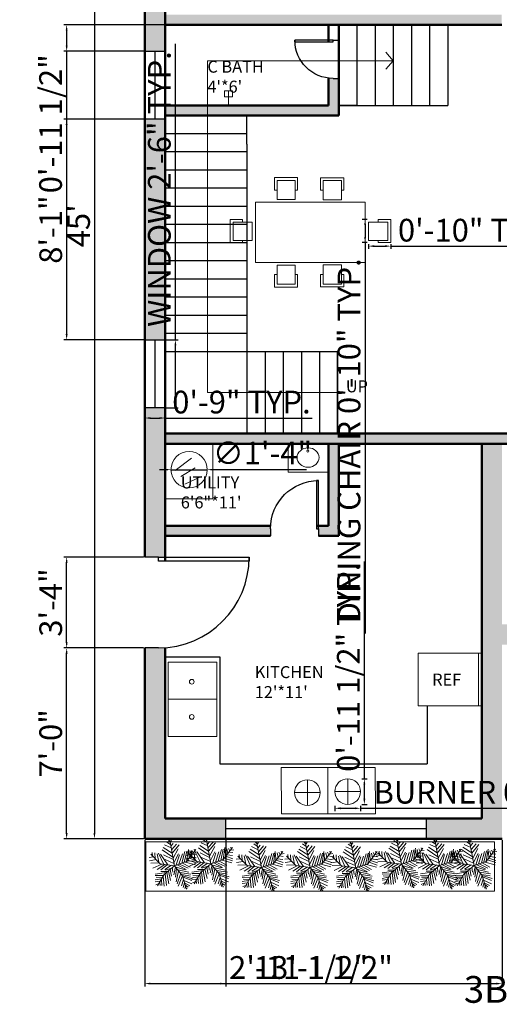
# Model space of a CAD drawing. Units: inches. Extents: x 772 to 1415, y 1573 to 2261.
# Tile 1 of 4: x 772 to 984, y 1573 to 2007. Entities that reach past the tile are written whole.
import ezdxf

# ---------------------------------------------------------------- set-up
doc = ezdxf.new("R2010")
doc.units = ezdxf.units.IN
for name, color, linetype, lineweight in [('A-ANNO-DIMS', 2, 'Continuous', 18), ('A-ANNO-SYMB', 7, 'Continuous', 18), ('A-ANNO-TEXT', 10, 'Continuous', 25), ('A-AREA-IDEN', 10, 'Continuous', 25), ('A-EQPM', 8, 'Continuous', 18), ('A-FLOR-FIXT', 9, 'Continuous', 18), ('A-FLOR-STRS', 7, 'Continuous', 25), ('A-FURN-FIXD', 210, 'Continuous', 25), ('A-WALL-PATT', 140, 'Continuous', 13), ('DOOR', 52, 'Continuous', 25), ('FUR', 210, 'Continuous', 18), ('L-PLNT-BEDS', 92, 'Continuous', 18), ('TREE', 92, 'Continuous', 13), ('WALL', 7, 'Continuous', 50), ('WINDOW', 80, 'Continuous', 25)]:
    doc.layers.add(name, color=color, linetype=linetype, lineweight=lineweight)
doc.styles.get("Standard").update_dxf_attribs({"font": 'arial.ttf'})
doc.dimstyles.new('ISO-25', dxfattribs={"dimtxt": 10, "dimasz": 2.5, "dimexe": 1.25, "dimexo": 0.625, "dimtad": 1, "dimdec": 0, "dimlunit": 4, "dimtxsty": 'Standard', "dimcen": 2.5, "dimadec": 0, "dimazin": 0, "dimtfac": 1, "dimtdec": 0, "dimtmove": 0, "dimatfit": 3, "dimfxl": 1, "dimarcsym": 0})

# ---------------------------------------------------------------- blocks, each defined once
blk = doc.blocks.new('*U2')
for p, q in [((0, 0), (0, -6)), ((40, 0), (40, -6))]:
    blk.add_line(p, q)
blk.add_lwpolyline([(0, 0), (0, 40), (1.75, 40), (1.75, 0)], close=True)
blk.add_arc((0, 0), 40, 0, 90)
blk = doc.blocks.new('*U6')
for p, q in [((-7.288, 39.707), (-21.778, 46.673)), ((-8.737, 47.138), (-17.069, 52.711)), ((-10.186, 53.64), (-13.084, 55.962)), ((0, 0), (-10.5, 57)), ((-9.099, 51.782), (-6.563, 55.962)), ((-7.65, 43.423), (-2.578, 49.46)), ((-5.839, 35.992), (4.667, 48.067)), ((-5.114, 27.632), (10.463, 46.673)), ((-31.5, 4.5), (-52.5, 25.5)), ((-48.585, 21.131), (-49.309, 29.026)), ((-43.513, 28.561), (-42.427, 15.558)), ((-38.442, 26.239), (-34.819, 7.663)), ((-35.544, 28.097), (-24.314, 3.947)), ((-14.533, 2.09), (-30.834, 25.31)), ((-3.665, 19.273), (-27.574, 35.527)), ((-5.114, 28.097), (-24.676, 40.636)), ((-24.314, 23.917), (-2.941, 13.7)), ((-2.941, 16.486), (8.652, 37.85)), ((-1.129, 6.734), (9.014, 26.704)), ((3.942, 1.625), (11.187, 24.381)), ((10.101, 3.483), (17.708, 26.239)), ((16.259, 5.805), (23.142, 31.348)), ((22.055, 7.198), (27.489, 32.277)), ((27, 9), (48, 36)), ((27.127, 9.056), (31.112, 35.992)), ((31.836, 30.883), (32.561, 16.486)), ((35.096, 32.741), (37.27, 22.524)), ((38.719, 34.134), (41.979, 28.561)), ((40.53, 25.775), (48.862, 24.846)), ((43.791, 29.954), (51.036, 30.883)), ((44.153, 36.456), (45.239, 32.741)), ((-47.498, 19.737), (-55.83, 18.344)), ((-40.615, 13.7), (-55.105, 10.913)), ((-33.37, 6.269), (-52.207, 5.34)), ((-28.299, 3.483), (-47.86, -5.805)), ((-21.416, 3.018), (-38.079, -8.128)), ((0, 0), (-31.5, 4.5)), ((-15.982, 2.09), (-30.11, -9.521)), ((0, 0), (-22.5, -19.5)), ((-6.563, 1.161), (-21.416, -8.128)), ((-20.691, 13.7), (-1.129, 4.876)), ((0, 0), (27, 9)), ((0, 0), (18, -22.5)), ((6.478, 1.625), (26.04, -8.592)), ((11.187, 3.483), (30.749, -5.805)), ((18.07, 5.805), (35.096, -3.483)), ((24.229, 7.663), (46.688, 1.625)), ((29.662, 12.307), (48.137, 6.269)), ((33.285, 16.486), (48.862, 10.913)), ((36.183, 19.737), (48.137, 17.88)), ((-17.431, -15.094), (-42.789, -18.809)), ((-24.314, -21.596), (-42.427, -22.06)), ((-22.5, -19.5), (-37.5, -45)), ((-15.257, -12.772), (-30.11, -12.772)), ((-20.691, -18.345), (-17.793, -44.352)), ((-6.563, -5.805), (-19.967, -9.985)), ((-17.069, -15.094), (-12.721, -40.172)), ((-13.446, -11.378), (-8.737, -32.741)), ((-9.461, -8.592), (-6.201, -23.453)), ((-4.752, -3.483), (-3.665, -14.629)), ((2.493, -3.019), (-1.491, -20.202)), ((1.769, -2.555), (24.229, -9.521)), ((5.029, -6.27), (2.131, -25.775)), ((9.014, -11.378), (3.58, -35.992)), ((14.085, -16.951), (6.478, -40.172)), ((7.565, -9.056), (32.198, -14.629)), ((12.274, -15.094), (36.907, -18.809)), ((16.259, -19.738), (36.183, -22.989)), ((-28.299, -29.026), (-42.789, -31.348)), ((-30.834, -34.135), (-42.427, -35.528)), ((-34.457, -39.708), (-40.978, -42.494)), ((-26.849, -26.24), (-40.253, -25.775)), ((-32.646, -36.921), (-31.921, -44.352)), ((-29.023, -30.884), (-27.936, -43.887)), ((-25.038, -23.918), (-22.865, -45.281)), ((18.07, -22.524), (8.289, -45.745)), ((20.244, -30.419), (15.897, -44.816)), ((18, -22.5), (27, -52.5)), ((18.433, -22.524), (40.53, -29.026)), ((19.157, -25.311), (38.719, -33.206)), ((22.78, -37.85), (19.519, -48.532)), ((21.331, -32.741), (39.081, -40.636)), ((22.78, -38.314), (34.372, -44.816)), ((24.591, -43.423), (30.749, -47.603)), ((24.591, -45.745), (23.142, -50.854)), ((26.764, -49.925), (28.213, -50.854))]:
    blk.add_line(p, q)
blk = doc.blocks.new('*D10')
at = {"layer": 'A-ANNO-DIMS', "color": 0, "lineweight": -2, "transparency": 16777216}
for p, q in [((827.03, 2185.98), (804.2, 2185.98)), ((805.45, 2183.48), (805.45, 1648.48)), ((827.03, 1645.98), (804.2, 1645.98))]:
    blk.add_line(p, q, dxfattribs=at)
at = {"layer": 'A-ANNO-DIMS', "color": 0, "transparency": 16777216}
for points in [[(805.04, 2183.48), (805.87, 2183.48), (805.45, 2185.98)], [(805.04, 1648.48), (805.87, 1648.48), (805.45, 1645.98)]]:
    blk.add_solid(points, dxfattribs=at)
at = {"layer": 'Defpoints', "color": 0, "transparency": 16777216}
for p in [(827.65, 2185.98), (805.45, 1645.98), (827.65, 1645.98)]:
    blk.add_point(p, dxfattribs=at)
at = {"layer": 'A-ANNO-DIMS', "color": 0, "transparency": 16777216, "insert": (799.74, 1915.98), "char_height": 10, "attachment_point": 5, "rotation": 90}
blk.add_mtext("45'", dxfattribs=at)
blk = doc.blocks.new('CHAIR-DINING')
for p, q in [((0, 4.23), (0, 9.75)), ((0, 9.75), (10.23, 9.75)), ((10.23, 9.75), (10.23, 4.23)), ((1.18, 4.23), (0, 4.23)), ((10.23, 4.23), (9.23, 4.23))]:
    blk.add_line(p, q)
blk.add_lwpolyline([(1.18, 0), (9.23, 0), (9.23, 8.46), (1.18, 8.46)], close=True)
blk = doc.blocks.new('WIN-88IN')
blk.add_line((0, 4.5), (88.26, 4.5))
blk.add_lwpolyline([(0, 9), (88.26, 9), (88.26, 0), (0, 0)], close=True)
blk = doc.blocks.new('WIN-30IN')
blk.add_line((4.5, 0), (4.5, 29.96))
blk.add_lwpolyline([(0, 29.96), (9, 29.96), (9, 0), (0, 0)], close=True)
blk = doc.blocks.new('COOKTOP-BURNER')
for p, q in [((5.65, 5.65), (5.65, 11.3)), ((5.65, 11.3), (5.65, 0)), ((11.3, 5.65), (0, 5.65)), ((5.65, 0), (5.65, 5.65)), ((5.65, 5.65), (11.3, 5.65))]:
    blk.add_line(p, q)
blk.add_circle((5.65, 5.65), 5.65)
blk = doc.blocks.new('*D25')
at = {"layer": 'A-ANNO-DIMS', "color": 0, "lineweight": -2, "transparency": 16777216}
for p, q in [((925.67, 1918.77), (923.51, 1918.77)), ((924.76, 1916.27), (924.76, 1911.03)), ((925.67, 1908.53), (923.51, 1908.53)), ((924.76, 1908.53), (924.76, 1736.44))]:
    blk.add_line(p, q, dxfattribs=at)
at = {"layer": 'A-ANNO-DIMS', "color": 0, "transparency": 16777216}
for points in [[(924.34, 1916.27), (925.17, 1916.27), (924.76, 1918.77)], [(924.34, 1911.03), (925.17, 1911.03), (924.76, 1908.53)]]:
    blk.add_solid(points, dxfattribs=at)
at = {"layer": 'Defpoints', "color": 0, "transparency": 16777216}
for p in [(926.29, 1918.77), (924.76, 1908.53), (926.29, 1908.53)]:
    blk.add_point(p, dxfattribs=at)
at = {"layer": 'A-ANNO-DIMS', "color": 0, "transparency": 16777216, "insert": (918.96, 1821.24), "char_height": 10, "attachment_point": 5, "rotation": 90}
blk.add_mtext('DINING CHAIR 0\'-10" TYP.', dxfattribs=at)
blk = doc.blocks.new('*D26')
at = {"layer": 'A-ANNO-DIMS', "color": 0, "lineweight": -2, "transparency": 16777216}
for p, q in [((926.29, 1907.91), (926.29, 1905.75)), ((928.79, 1907), (933.54, 1907)), ((936.04, 1907.91), (936.04, 1905.75)), ((936.04, 1907), (1008.52, 1907))]:
    blk.add_line(p, q, dxfattribs=at)
at = {"layer": 'A-ANNO-DIMS', "color": 0, "transparency": 16777216}
for points in [[(928.79, 1907.42), (928.79, 1906.58), (926.29, 1907)], [(933.54, 1907.42), (933.54, 1906.58), (936.04, 1907)]]:
    blk.add_solid(points, dxfattribs=at)
at = {"layer": 'Defpoints', "color": 0, "transparency": 16777216}
for p in [(926.29, 1908.53), (936.04, 1908.53), (936.04, 1907)]:
    blk.add_point(p, dxfattribs=at)
at = {"layer": 'A-ANNO-DIMS', "color": 0, "transparency": 16777216, "insert": (973.53, 1912.73), "char_height": 10, "attachment_point": 5}
blk.add_mtext('0\'-10" TYP.', dxfattribs=at)
blk = doc.blocks.new('*D35')
at = {"layer": 'A-ANNO-DIMS', "color": 0, "lineweight": -2, "transparency": 16777216}
for p, q in [((841.15, 1865.74), (841.15, 1996.03)), ((837.28, 1865.74), (842.4, 1865.74)), ((841.15, 1838.28), (841.15, 1863.24)), ((837.28, 1835.78), (842.4, 1835.78))]:
    blk.add_line(p, q, dxfattribs=at)
at = {"layer": 'A-ANNO-DIMS', "color": 0, "transparency": 16777216}
for points in [[(840.73, 1863.24), (841.56, 1863.24), (841.15, 1865.74)], [(840.73, 1838.28), (841.56, 1838.28), (841.15, 1835.78)]]:
    blk.add_solid(points, dxfattribs=at)
at = {"layer": 'Defpoints', "color": 0, "transparency": 16777216}
for p in [(836.65, 1865.74), (841.15, 1865.74), (836.65, 1835.78)]:
    blk.add_point(p, dxfattribs=at)
at = {"layer": 'A-ANNO-DIMS', "color": 0, "transparency": 16777216, "insert": (835.35, 1932.14), "char_height": 10, "attachment_point": 5, "rotation": 90}
blk.add_mtext('WINDOW 2\'-6" TYP.', dxfattribs=at)
blk = doc.blocks.new('*D36')
at = {"layer": 'A-ANNO-DIMS', "color": 0, "lineweight": -2, "transparency": 16777216}
for p, q in [((827.65, 1835.15), (827.65, 1830.04)), ((836.65, 1835.15), (836.65, 1830.04)), ((830.15, 1831.29), (834.15, 1831.29)), ((836.65, 1831.29), (901.36, 1831.29))]:
    blk.add_line(p, q, dxfattribs=at)
at = {"layer": 'A-ANNO-DIMS', "color": 0, "transparency": 16777216}
for points in [[(830.15, 1831.7), (830.15, 1830.87), (827.65, 1831.29)], [(834.15, 1831.7), (834.15, 1830.87), (836.65, 1831.29)]]:
    blk.add_solid(points, dxfattribs=at)
at = {"layer": 'Defpoints', "color": 0, "transparency": 16777216}
for p in [(827.65, 1835.78), (836.65, 1835.78), (836.65, 1831.29)]:
    blk.add_point(p, dxfattribs=at)
at = {"layer": 'A-ANNO-DIMS', "color": 0, "transparency": 16777216, "insert": (870.25, 1837.02), "char_height": 10, "attachment_point": 5}
blk.add_mtext('0\'-9" TYP.', dxfattribs=at)
blk = doc.blocks.new('*D39')
at = {"layer": 'A-ANNO-DIMS', "color": 0, "lineweight": -2, "transparency": 16777216}
for p, q in [((911.44, 1660.47), (911.44, 1658.15)), ((913.94, 1659.4), (920.23, 1659.4)), ((922.73, 1660.47), (922.73, 1658.15)), ((922.73, 1659.4), (1080.94, 1659.4))]:
    blk.add_line(p, q, dxfattribs=at)
at = {"layer": 'A-ANNO-DIMS', "color": 0, "transparency": 16777216}
for points in [[(913.94, 1659.82), (913.94, 1658.99), (911.44, 1659.4)], [(920.23, 1659.82), (920.23, 1658.99), (922.73, 1659.4)]]:
    blk.add_solid(points, dxfattribs=at)
at = {"layer": 'Defpoints', "color": 0, "transparency": 16777216}
for p in [(911.44, 1661.1), (922.73, 1661.1), (922.73, 1659.4)]:
    blk.add_point(p, dxfattribs=at)
at = {"layer": 'A-ANNO-DIMS', "color": 0, "transparency": 16777216, "insert": (1003.09, 1665.2), "char_height": 10, "attachment_point": 5}
blk.add_mtext('BURNER 0\'-11 1/2" TYP.', dxfattribs=at)
blk = doc.blocks.new('*D40')
at = {"layer": 'A-ANNO-DIMS', "color": 0, "lineweight": -2, "transparency": 16777216}
for p, q in [((924.43, 1672.4), (924.43, 1768.17)), ((923.36, 1672.4), (925.68, 1672.4)), ((924.43, 1663.6), (924.43, 1669.9)), ((923.36, 1661.1), (925.68, 1661.1))]:
    blk.add_line(p, q, dxfattribs=at)
at = {"layer": 'A-ANNO-DIMS', "color": 0, "transparency": 16777216}
for points in [[(924.01, 1669.9), (924.85, 1669.9), (924.43, 1672.4)], [(924.01, 1663.6), (924.85, 1663.6), (924.43, 1661.1)]]:
    blk.add_solid(points, dxfattribs=at)
at = {"layer": 'Defpoints', "color": 0, "transparency": 16777216}
for p in [(922.73, 1672.4), (924.43, 1672.4), (922.73, 1661.1)]:
    blk.add_point(p, dxfattribs=at)
at = {"layer": 'A-ANNO-DIMS', "color": 0, "transparency": 16777216, "insert": (918.63, 1721.54), "char_height": 10, "attachment_point": 5, "rotation": 90}
blk.add_mtext('0\'-11 1/2" TYP.', dxfattribs=at)
blk = doc.blocks.new('*D41')
at = {"layer": 'A-ANNO-DIMS', "color": 0, "lineweight": -2, "transparency": 16777216}
for p, q in [((827.65, 1645.36), (827.65, 1580.94)), ((985.15, 1645.36), (985.15, 1580.94)), ((830.15, 1582.19), (982.65, 1582.19))]:
    blk.add_line(p, q, dxfattribs=at)
at = {"layer": 'A-ANNO-DIMS', "color": 0, "transparency": 16777216}
for points in [[(830.15, 1582.61), (830.15, 1581.78), (827.65, 1582.19)], [(982.65, 1582.61), (982.65, 1581.78), (985.15, 1582.19)]]:
    blk.add_solid(points, dxfattribs=at)
at = {"layer": 'Defpoints', "color": 0, "transparency": 16777216}
for p in [(827.65, 1645.98), (985.15, 1645.98), (985.15, 1582.19)]:
    blk.add_point(p, dxfattribs=at)
at = {"layer": 'A-ANNO-DIMS', "color": 0, "transparency": 16777216, "insert": (906.4, 1587.99), "char_height": 10, "attachment_point": 5}
blk.add_mtext('13\'-1 1/2"', dxfattribs=at)
blk = doc.blocks.new('*D52')
at = {"layer": 'A-ANNO-DIMS', "color": 0, "lineweight": -2, "transparency": 16777216}
for p, q in [((836.03, 2004.48), (791.95, 2004.48)), ((793.2, 2001.98), (793.2, 1995.35)), ((827.03, 1992.85), (791.95, 1992.85)), ((793.2, 1992.85), (793.2, 1931.44))]:
    blk.add_line(p, q, dxfattribs=at)
at = {"layer": 'A-ANNO-DIMS', "color": 0, "transparency": 16777216}
for points in [[(792.78, 2001.98), (793.62, 2001.98), (793.2, 2004.48)], [(792.78, 1995.35), (793.62, 1995.35), (793.2, 1992.85)]]:
    blk.add_solid(points, dxfattribs=at)
at = {"layer": 'Defpoints', "color": 0, "transparency": 16777216}
for p in [(836.65, 2004.48), (793.2, 1992.85), (827.65, 1992.85)]:
    blk.add_point(p, dxfattribs=at)
at = {"layer": 'A-ANNO-DIMS', "color": 0, "transparency": 16777216, "insert": (787.4, 1960.9), "char_height": 10, "attachment_point": 5, "rotation": 90}
blk.add_mtext('0\'-11 1/2"', dxfattribs=at)
blk = doc.blocks.new('*D53')
at = {"layer": 'A-ANNO-DIMS', "color": 0, "lineweight": -2, "transparency": 16777216}
for p, q in [((827.03, 1962.89), (791.95, 1962.89)), ((793.2, 1960.39), (793.2, 1868.24)), ((827.03, 1865.74), (791.95, 1865.74))]:
    blk.add_line(p, q, dxfattribs=at)
at = {"layer": 'A-ANNO-DIMS', "color": 0, "transparency": 16777216}
for points in [[(792.78, 1960.39), (793.62, 1960.39), (793.2, 1962.89)], [(792.78, 1868.24), (793.62, 1868.24), (793.2, 1865.74)]]:
    blk.add_solid(points, dxfattribs=at)
at = {"layer": 'Defpoints', "color": 0, "transparency": 16777216}
for p in [(827.65, 1962.89), (793.2, 1865.74), (827.65, 1865.74)]:
    blk.add_point(p, dxfattribs=at)
at = {"layer": 'A-ANNO-DIMS', "color": 0, "transparency": 16777216, "insert": (787.47, 1914.31), "char_height": 10, "attachment_point": 5, "rotation": 90}
blk.add_mtext('8\'-1"', dxfattribs=at)
blk = doc.blocks.new('*D54')
at = {"layer": 'A-ANNO-DIMS', "color": 0, "lineweight": -2, "transparency": 16777216}
for p, q in [((827.65, 1645.36), (827.65, 1580.94)), ((863.4, 1645.36), (863.4, 1580.94)), ((830.15, 1582.19), (860.9, 1582.19)), ((863.4, 1582.19), (924.97, 1582.19))]:
    blk.add_line(p, q, dxfattribs=at)
at = {"layer": 'A-ANNO-DIMS', "color": 0, "transparency": 16777216}
for points in [[(830.15, 1582.61), (830.15, 1581.78), (827.65, 1582.19)], [(860.9, 1582.61), (860.9, 1581.78), (863.4, 1582.19)]]:
    blk.add_solid(points, dxfattribs=at)
at = {"layer": 'Defpoints', "color": 0, "transparency": 16777216}
for p in [(827.65, 1645.98), (863.4, 1645.98), (863.4, 1582.19)]:
    blk.add_point(p, dxfattribs=at)
at = {"layer": 'A-ANNO-DIMS', "color": 0, "transparency": 16777216, "insert": (895.44, 1587.99), "char_height": 10, "attachment_point": 5}
blk.add_mtext('2\'-11 1/2"', dxfattribs=at)
blk = doc.blocks.new('*D57')
at = {"layer": 'A-ANNO-DIMS', "color": 0, "lineweight": -2, "transparency": 16777216}
for p, q in [((827.03, 1730.04), (791.95, 1730.04)), ((793.2, 1648.48), (793.2, 1727.54)), ((827.03, 1645.98), (791.95, 1645.98))]:
    blk.add_line(p, q, dxfattribs=at)
at = {"layer": 'A-ANNO-DIMS', "color": 0, "transparency": 16777216}
for points in [[(792.78, 1727.54), (793.62, 1727.54), (793.2, 1730.04)], [(792.78, 1648.48), (793.62, 1648.48), (793.2, 1645.98)]]:
    blk.add_solid(points, dxfattribs=at)
at = {"layer": 'Defpoints', "color": 0, "transparency": 16777216}
for p in [(793.2, 1730.04), (827.65, 1730.04), (827.65, 1645.98)]:
    blk.add_point(p, dxfattribs=at)
at = {"layer": 'A-ANNO-DIMS', "color": 0, "transparency": 16777216, "insert": (787.47, 1688.01), "char_height": 10, "attachment_point": 5, "rotation": 90}
blk.add_mtext('7\'-0"', dxfattribs=at)
blk = doc.blocks.new('*D58')
at = {"layer": 'A-ANNO-DIMS', "color": 0, "lineweight": -2, "transparency": 16777216}
for p, q in [((827.03, 1770.04), (791.95, 1770.04)), ((793.2, 1732.54), (793.2, 1767.54)), ((827.03, 1730.04), (791.95, 1730.04))]:
    blk.add_line(p, q, dxfattribs=at)
at = {"layer": 'A-ANNO-DIMS', "color": 0, "transparency": 16777216}
for points in [[(792.78, 1767.54), (793.62, 1767.54), (793.2, 1770.04)], [(792.78, 1732.54), (793.62, 1732.54), (793.2, 1730.04)]]:
    blk.add_solid(points, dxfattribs=at)
at = {"layer": 'Defpoints', "color": 0, "transparency": 16777216}
for p in [(793.2, 1770.04), (827.65, 1770.04), (827.65, 1730.04)]:
    blk.add_point(p, dxfattribs=at)
at = {"layer": 'A-ANNO-DIMS', "color": 0, "transparency": 16777216, "insert": (787.47, 1750.04), "char_height": 10, "attachment_point": 5, "rotation": 90}
blk.add_mtext('3\'-4"', dxfattribs=at)
blk = doc.blocks.new('*D67')
at = {"layer": 'A-ANNO-DIMS', "color": 0, "lineweight": -2, "transparency": 16777216}
for p, q in [((836.67, 1808.54), (834.17, 1808.54)), ((839.17, 1808.54), (855.18, 1808.54)), ((898.89, 1808.54), (857.68, 1808.54))]:
    blk.add_line(p, q, dxfattribs=at)
at = {"layer": 'A-ANNO-DIMS', "color": 0, "transparency": 16777216}
for points in [[(836.67, 1808.96), (836.67, 1808.13), (839.17, 1808.54)], [(857.68, 1808.96), (857.68, 1808.13), (855.18, 1808.54)]]:
    blk.add_solid(points, dxfattribs=at)
at = {"layer": 'Defpoints', "color": 0, "transparency": 16777216}
for p in [(839.17, 1808.54), (855.18, 1808.54)]:
    blk.add_point(p, dxfattribs=at)
at = {"layer": 'A-ANNO-DIMS', "color": 0, "transparency": 16777216, "insert": (879.53, 1814.55), "char_height": 10, "attachment_point": 5, "rotation": 359.9994}
blk.add_mtext('∅1\'-4"', dxfattribs=at)

msp = doc.modelspace()

# ---------------------------------------------------------------- hatches: boundary and pattern name
at = {"layer": 'A-WALL-PATT'}
h = msp.add_hatch(color=256, dxfattribs=at)
h.dxf.hatch_style = 1
h.paths.add_polyline_path([(885.72, 2185.98), (827.65, 2185.98), (827.65, 1992.85), (836.65, 1992.85), (836.65, 2176.98), (885.72, 2176.98)])
h.paths.add_polyline_path([(1050.98, 2185.98), (977.81, 2185.98), (977.81, 2176.98), (1028.65, 2176.98), (1050.98, 2176.98)])
h.paths.add_polyline_path([(1112.88, 2185.98), (1085.61, 2185.98), (1085.61, 2176.98), (1105.15, 2176.98), (1112.88, 2176.98)])
h.paths.add_polyline_path([(1192.68, 2185.98), (1147.51, 2185.98), (1147.51, 2176.98), (1181.65, 2176.98), (1192.68, 2176.98)])
h.paths.add_polyline_path([(1307.65, 2185.98), (1284.78, 2185.98), (1284.78, 2176.98), (1298.65, 2176.98), (1298.65, 1819.98), (1307.65, 1819.98)])
h.paths.add_polyline_path([(1033.15, 2176.98), (1028.65, 2176.98), (1028.65, 2036.41), (1032.25, 2036.41, -0.009373), (1033.15, 2036.4)])
h.paths.add_polyline_path([(1036.22, 2092.98), (1033.15, 2092.98), (1033.15, 2088.48), (1036.22, 2088.48)])
h.paths.add_polyline_path([(1154.65, 2104.98), (1135.16, 2104.98, -0.008763), (1135.17, 2104.13), (1135.17, 2100.48), (1154.65, 2100.48)])
h.paths.add_polyline_path([(1159.15, 2176.98), (1154.65, 2176.98), (1154.65, 2051.78), (1159.15, 2051.78)])
h.paths.add_polyline_path([(914.37, 1839.72), (927.25, 1839.72), (927.25, 1850.6), (914.37, 1850.6)], flags=9)
h.paths.add_polyline_path([(1081.37, 1890.08), (1108.45, 1890.08), (1108.45, 1909.77), (1081.37, 1909.77)], flags=9)
h.paths.add_polyline_path([(1220.18, 1938.14), (1269.92, 1938.14), (1269.92, 1957.83), (1220.18, 1957.83)], flags=9)
h.paths.add_polyline_path([(1219.66, 2046.23), (1263.24, 2046.23), (1263.24, 2065.92), (1219.66, 2065.92)], flags=9)
h.paths.add_polyline_path([(1107.96, 2127.66), (1143.78, 2127.66), (1143.78, 2147.35), (1107.96, 2147.35)], flags=9)
h.paths.add_polyline_path([(1040.84, 2046.02), (1081.99, 2046.02), (1081.99, 2065.72), (1040.84, 2065.72)], flags=9)
h.paths.add_polyline_path([(1051.44, 2131.75), (1073.61, 2131.75), (1073.61, 2151.44), (1051.44, 2151.44)], flags=9)
h.paths.add_polyline_path([(953.87, 2096.26), (1003.05, 2096.26), (1003.05, 2115.95), (953.87, 2115.95)], flags=9)
h = msp.add_hatch(color=256, dxfattribs=at)
h.dxf.hatch_style = 1
h.paths.add_polyline_path([(836.65, 1835.78), (827.65, 1835.78), (827.65, 1770.04), (833.65, 1770.04), (836.65, 1770.04)])
h.paths.add_polyline_path([(1154.65, 1824.48), (938.65, 1824.48), (836.65, 1824.48), (836.65, 1819.98), (980.65, 1819.98), (1154.65, 1819.98)])
h.paths.add_polyline_path([(836.65, 1962.89), (827.65, 1962.89), (827.65, 1865.74), (836.65, 1865.74)])
h.paths.add_polyline_path([(913.15, 1980.86), (910.62, 1980.86, -0.029352), (908.65, 1980.98), (908.65, 1968.98), (900.27, 1968.98), (855.22, 1968.98), (855.22, 1964.48), (913.15, 1964.48)])
h.paths.add_polyline_path([(855.22, 1968.98), (836.65, 1968.98), (836.65, 1964.48), (855.22, 1964.48)])
h.paths.add_polyline_path([(984.95, 2008.98), (836.65, 2008.98), (836.65, 2004.48), (908.65, 2004.48), (984.95, 2004.48)])
h.paths.add_polyline_path([(1298.65, 2008.98), (1171.7, 2008.98), (1154.65, 2008.98), (1154.65, 2004.48), (1298.65, 2004.48)])
h.paths.add_polyline_path([(1159.15, 2011.78), (1154.65, 2011.78), (1154.65, 2008.98), (1159.15, 2008.98)])
h.paths.add_polyline_path([(1159.15, 2004.48), (1154.65, 2004.48), (1154.65, 1998.53), (1159.15, 1998.53)])
h = msp.add_hatch(color=256, dxfattribs=at)
h.dxf.hatch_style = 1
h.paths.add_polyline_path([(863.4, 1654.98), (836.65, 1654.98), (836.65, 1678.98), (836.65, 1730.15, -0.01877), (833.65, 1730.04), (827.65, 1730.04), (827.65, 1645.98), (863.4, 1645.98)])
h.paths.add_polyline_path([(985.15, 1654.98), (985.15, 1819.98), (976.15, 1819.98), (976.15, 1654.98), (951.66, 1654.98), (951.66, 1645.98), (985.15, 1645.98)])
h.paths.add_polyline_path([(989, 1737.48), (989, 1740.48), (985.15, 1740.48), (985.15, 1731.48), (989, 1731.48)])
h.paths.add_polyline_path([(1045.2, 1740.48), (1028.89, 1740.48, -0.01877), (1029, 1737.48), (1029, 1731.48), (1045.2, 1731.48)])
h.paths.add_polyline_path([(1145.65, 1819.98), (1136.65, 1819.98), (1136.65, 1740.48), (1133.46, 1740.48), (1133.46, 1731.48), (1145.65, 1731.48)])
h = msp.add_hatch(color=256, dxfattribs=at)
h.dxf.hatch_style = 1
h.paths.add_polyline_path([(883.08, 1783.87), (836.65, 1783.87), (836.65, 1779.37), (883.04, 1779.37), (883.04, 1782.55, -0.015579)])
h.paths.add_polyline_path([(913.15, 1819.98), (908.65, 1819.98), (908.65, 1807.38), (908.65, 1783.87), (904.24, 1783.87), (904.24, 1782.55), (904.24, 1779.37), (913.15, 1779.37)])

# ---------------------------------------------------------------- linework, layer by layer
at = {"layer": 'A-ANNO-SYMB'}
for p, q in [((937.15, 1988.68), (933.87, 1992.46)), ((855.22, 1842.48), (855.22, 1988.68)), ((855.22, 1988.68), (937.15, 1988.68)), ((937.15, 1988.68), (933.87, 1984.9)), ((912.63, 1842.48), (855.22, 1842.48))]:
    msp.add_line(p, q, dxfattribs=at)
at = {"layer": 'A-EQPM'}
for p, q in [((841.01, 1808.21), (848.29, 1813.6)), ((843.51, 1805.55), (849.84, 1809.43)), ((845.29, 1802.11), (852.51, 1805.6)), ((974.79, 1727.66), (974.79, 1704.52)), ((908.3, 1677.32), (908.3, 1656.94))]:
    msp.add_line(p, q, dxfattribs=at)
for points in [[(836.65, 1819.98), (857.6, 1819.98), (857.6, 1795.77), (836.65, 1795.77)], [(976.15, 1727.66), (948.12, 1727.66), (948.12, 1704.52), (976.15, 1704.52)], [(887.81, 1677.32), (929.23, 1677.32), (929.28, 1656.94), (887.86, 1656.94)]]:
    msp.add_lwpolyline(points, close=True, dxfattribs=at)
msp.add_circle((847.18, 1808.54), 8, dxfattribs=at)
at = {"layer": 'A-FLOR-FIXT'}
for p, q in [((864.52, 1975.46), (864.52, 1968.98)), ((837.9, 1707.4), (859.33, 1707.4))]:
    msp.add_line(p, q, dxfattribs=at)
for points in [[(862.75, 1972.76), (866.28, 1972.76), (866.28, 1975.46), (862.75, 1975.46)], [(908.65, 1819.98), (890.87, 1819.98), (890.87, 1807.38), (908.65, 1807.38)], [(837.9, 1723.81), (859.33, 1723.81), (859.33, 1691), (837.9, 1691)]]:
    msp.add_lwpolyline(points, close=True, dxfattribs=at)
for centre, radius in [((899.53, 1816.76), 0.441), ((848.37, 1715.15), 1.03), ((848.37, 1699.63), 1.03)]:
    msp.add_circle(centre, radius, dxfattribs=at)
msp.add_ellipse((899.64, 1813.89), major_axis=(4.86, 0), ratio=0.875, dxfattribs=at)
at = {"layer": 'A-FLOR-STRS'}
for p, q in [((921.15, 2004.48), (921.15, 1968.98)), ((929.15, 2004.48), (929.15, 1968.98)), ((937.15, 2004.48), (937.15, 1968.98)), ((945.15, 2004.48), (945.15, 1968.98)), ((953.15, 2004.48), (953.15, 1968.98)), ((961.15, 2004.48), (961.15, 1968.98)), ((921.15, 1968.98), (913.15, 1968.98)), ((913.15, 1968.98), (961.15, 1968.98)), ((872.65, 1964.48), (836.65, 1964.48)), ((872.65, 1951.98), (872.65, 1964.48)), ((872.65, 1956.48), (836.65, 1956.48)), ((872.65, 1951.98), (872.65, 1860.48)), ((872.65, 1948.48), (836.65, 1948.48)), ((872.65, 1940.48), (836.65, 1940.48)), ((872.65, 1932.48), (836.65, 1932.48)), ((872.65, 1924.48), (836.65, 1924.48)), ((872.65, 1916.48), (836.65, 1916.48)), ((872.65, 1908.48), (836.65, 1908.48)), ((872.65, 1900.48), (836.65, 1900.48)), ((872.65, 1892.48), (836.65, 1892.48)), ((872.65, 1884.48), (836.65, 1884.48)), ((872.65, 1876.48), (836.65, 1876.48)), ((872.65, 1868.48), (836.65, 1868.48)), ((872.65, 1860.48), (836.65, 1860.48)), ((912.63, 1860.48), (872.65, 1860.48)), ((872.65, 1860.48), (872.65, 1824.48)), ((880.65, 1860.48), (880.65, 1824.48)), ((888.65, 1860.48), (888.65, 1824.48)), ((896.65, 1860.48), (896.65, 1824.48)), ((904.65, 1860.48), (904.65, 1824.48)), ((912.63, 1824.48), (912.63, 1860.48)), ((912.65, 1860.48), (912.65, 1824.48))]:
    msp.add_line(p, q, dxfattribs=at)
at = {"layer": 'A-FURN-FIXD'}
for p, q in [((836.65, 1726.06), (836.65, 1726.06)), ((836.65, 1726.06), (860.65, 1726.06)), ((860.65, 1726.06), (860.65, 1678.98)), ((952.15, 1704.52), (952.15, 1678.98)), ((836.65, 1654.98), (836.65, 1678.98)), ((860.65, 1678.98), (952.15, 1678.98))]:
    msp.add_line(p, q, dxfattribs=at)
at = {"layer": 'FUR'}
msp.add_lwpolyline([(876.47, 1926.34), (924.81, 1926.34), (924.81, 1899.83), (876.47, 1899.83)], close=True, dxfattribs=at)
at = {"layer": 'L-PLNT-BEDS'}
msp.add_lwpolyline([(828.15, 1644.58), (981.82, 1644.58), (981.82, 1622.85), (828.15, 1622.85)], close=True, dxfattribs=at)
at = {"layer": 'WALL'}
for p, q in [((827.65, 1770.04), (827.65, 2185.98)), ((836.65, 1768.29), (836.65, 2176.98)), ((836.65, 2004.48), (908.65, 2004.48)), ((984.95, 2004.48), (836.65, 2004.48)), ((908.65, 1999.98), (908.65, 2004.48)), ((913.15, 1999.98), (913.15, 2004.48)), ((908.65, 1999.98), (908.65, 1996.97)), ((913.15, 1999.98), (913.15, 1997.71)), ((913.15, 1999.98), (913.15, 1964.48)), ((908.65, 1968.98), (908.65, 1980.98)), ((913.15, 1968.98), (913.15, 1980.86)), ((900.27, 1968.98), (836.65, 1968.98)), ((908.65, 1968.98), (900.27, 1968.98)), ((913.15, 1969.61), (913.15, 1966.48)), ((913.15, 1964.48), (913.15, 1968.98)), ((913.15, 1964.48), (836.65, 1964.48)), ((938.65, 1824.48), (836.65, 1824.48)), ((1154.65, 1824.48), (938.65, 1824.48)), ((1154.65, 1819.98), (836.65, 1819.98)), ((836.65, 1819.98), (980.65, 1819.98)), ((836.65, 1819.98), (836.65, 1783.98)), ((908.65, 1783.87), (908.65, 1819.98)), ((913.15, 1779.37), (913.15, 1819.98)), ((976.15, 1819.98), (976.15, 1654.98)), ((836.65, 1783.87), (883.08, 1783.87)), ((903.31, 1783.87), (908.65, 1783.87)), ((836.65, 1779.37), (883.04, 1779.37)), ((904.24, 1779.37), (913.15, 1779.37)), ((827.65, 1645.98), (827.65, 1730.04)), ((836.65, 1654.98), (836.65, 1730.15)), ((976.15, 1654.98), (836.65, 1654.98)), ((985.15, 1645.98), (827.65, 1645.98))]:
    msp.add_line(p, q, dxfattribs=at)

# ---------------------------------------------------------------- block references
at = {"layer": 'A-EQPM'}
for p in [(893.66, 1660.67), (911.44, 1661.1)]:
    msp.add_blockref('COOKTOP-BURNER', p, dxfattribs=at)
at = {"layer": 'DOOR', "xscale": -0.42118038010609, "yscale": 0.42118038010609, "zscale": 0.42118038010609, "rotation": 90}
msp.add_blockref('*U2', (910.62, 1997.71), dxfattribs=at)
at = {"layer": 'DOOR', "xscale": -0.5299835864931757, "yscale": 0.5299835864931757, "zscale": 0.5299835864931757}
msp.add_blockref('*U2', (904.24, 1782.55), dxfattribs=at)
at = {"layer": 'DOOR', "rotation": 270}
msp.add_blockref('*U2', (833.65, 1770.04), dxfattribs=at)
at = {"layer": 'FUR'}
for p in [(884.75, 1927.48), (905.12, 1927.39)]:
    msp.add_blockref('CHAIR-DINING', p, dxfattribs=at)
at = {"layer": 'FUR', "extrusion": (0, 0, -1), "zscale": -1}
for p, rotation in [((-874.99, 1918.77), 270.0000000000017), ((-884.75, 1898.69), 180), ((-905.12, 1898.77), 180)]:
    msp.add_blockref('CHAIR-DINING', p, dxfattribs=dict(at, rotation=rotation))
at = {"layer": 'FUR', "rotation": 270.000000000001}
msp.add_blockref('CHAIR-DINING', (926.29, 1918.77), dxfattribs=at)
at = {"layer": 'TREE', "xscale": 0.198069497027702, "yscale": 0.198069497027702, "zscale": 0.198069497027702}
for p in [(840.69, 1634.12), (856.8, 1635.01), (879.02, 1633.31), (900.47, 1633.31), (920.6, 1633.18), (940.74, 1634.75), (957.6, 1634.23), (972.77, 1634.23)]:
    msp.add_blockref('*U6', p, dxfattribs=at)
at = {"layer": 'WINDOW'}
for name, p in [('WIN-30IN', (827.65, 1962.89)), ('WIN-30IN', (827.65, 1835.78)), ('WIN-88IN', (863.4, 1645.98))]:
    msp.add_blockref(name, p, dxfattribs=at)

# ---------------------------------------------------------------- texts
at = {"layer": 'A-ANNO-TEXT', "attachment_point": 1}
for s, width, gutter_width, insert, char_height in [('UP', 83.1931, 26.39, (916.27, 1847.88), 5.277), ('REF', 83.1931, 26.39, (954.31, 1718.74), 5.277), ('3BHK HOUSE PLAN', 1239.311, 58.94, (968.3, 1585.54), 11.7878)]:
    msp.add_mtext_dynamic_manual_height_columns(s, width=width, gutter_width=gutter_width, heights=[0], dxfattribs=dict(at, insert=insert, char_height=char_height))
at = {"layer": 'A-AREA-IDEN', "char_height": 5.277, "attachment_point": 1}
for s, insert in [("C BATH\\P4'*6'", (855.22, 1988.68)), ('UTILITY\\P6\'6"*11\'', (843.51, 1805.55)), ("KITCHEN\\P12'*11'", (876.11, 1722.02))]:
    msp.add_mtext_dynamic_manual_height_columns(s, width=83.1931, gutter_width=26.39, heights=[0], dxfattribs=dict(at, insert=insert))

# ---------------------------------------------------------------- dimensions: what is measured, and where the dimension line sits
at = {"layer": 'A-ANNO-DIMS'}
for base, p1, p2, override, picture, middle in [((805.45, 1645.98), (827.65, 2185.98), (827.65, 1645.98), {"dimclrd": 0, "dimclre": 0, "dimclrt": 0}, '*D10', (799.74, 1915.98)), ((793.2, 1992.85), (836.65, 2004.48), (827.65, 1992.85), {"dimdec": 1, "dimlfac": 1, "dimrnd": 0, "dimzin": 1, "dimdsep": 46, "dimlunit": 4, "dimfrac": 2}, '*D52', (787.4, 1960.9)), ((793.1995, 1865.7405), (827.6509, 1962.8864), (827.6509, 1865.7405), {"dimdec": 1, "dimlfac": 1, "dimrnd": 0, "dimzin": 1, "dimdsep": 46, "dimlunit": 4, "dimfrac": 2}, '*D53', (787.4687, 1914.3134)), ((793.2, 1770.04), (827.65, 1730.04), (827.65, 1770.04), {"dimdec": 1, "dimlfac": 1, "dimrnd": 0, "dimzin": 1, "dimdsep": 46, "dimlunit": 4, "dimfrac": 2}, '*D58', (787.47, 1750.04)), ((793.2, 1730.04), (827.65, 1645.98), (827.65, 1730.04), {"dimdec": 1, "dimlfac": 1, "dimrnd": 0, "dimzin": 1, "dimdsep": 46, "dimlunit": 4, "dimfrac": 2}, '*D57', (787.47, 1688.01))]:
    dim = msp.add_linear_dim(base=base, p1=p1, p2=p2, angle=90, dimstyle='ISO-25', override=override, dxfattribs=at)
    dim.commit()
    dim.dimension.update_dxf_attribs({"geometry": picture, "text_midpoint": middle})
for base, p1, p2, angle, text, picture, middle in [((841.15, 1865.74), (836.65, 1835.78), (836.65, 1865.74), 90, 'WINDOW <> TYP.', '*D35', (835.35, 1932.14)), ((936.0429, 1906.9998), (926.2923, 1908.5349), (936.0429, 1908.5349), 0, '<> TYP.', '*D26', (973.5302, 1912.7305)), ((924.76, 1908.53), (926.29, 1918.77), (926.29, 1908.53), 270, 'DINING CHAIR <> TYP.', '*D25', (918.96, 1821.24)), ((924.43, 1672.4), (922.73, 1661.1), (922.73, 1672.4), 90, '<> TYP.', '*D40', (918.63, 1721.54))]:
    dim = msp.add_linear_dim(base=base, p1=p1, p2=p2, angle=angle, text=text, dimstyle='ISO-25', override={"dimdec": 1, "dimlfac": 1, "dimrnd": 0, "dimzin": 1, "dimdsep": 46, "dimlunit": 4, "dimfrac": 2}, dxfattribs=at)
    dim.commit()
    dim.dimension.update_dxf_attribs({"geometry": picture, "text_midpoint": middle})
for base, p1, p2, text, picture, middle in [((836.65, 1831.29), (827.65, 1835.78), (836.65, 1835.78), '<> TYP.', '*D36', (870.25, 1837.02)), ((922.73, 1659.4), (911.44, 1661.1), (922.73, 1661.1), 'BURNER <> TYP.', '*D39', (1003.09, 1665.2))]:
    dim = msp.add_linear_dim(base=base, p1=p1, p2=p2, text=text, dimstyle='ISO-25', override={"dimdec": 1, "dimlfac": 1, "dimrnd": 0, "dimzin": 1, "dimdsep": 46, "dimlunit": 4, "dimfrac": 2}, dxfattribs=at)
    dim.commit()
    dim.dimension.update_dxf_attribs({"geometry": picture, "text_midpoint": middle})
dim = msp.add_diameter_dim_2p(p1=(839.17, 1808.54), p2=(855.18, 1808.54), dimstyle='ISO-25', override={"dimdec": 1, "dimlfac": 1, "dimrnd": 0, "dimzin": 1, "dimdsep": 46, "dimlunit": 4, "dimfrac": 2}, dxfattribs=at)
dim.commit()
dim.dimension.update_dxf_attribs({"geometry": '*D67', "text_midpoint": (879.53, 1808.54), "dimtype": 163})
for base, p1, p2, picture, middle in [((985.15, 1582.19), (827.65, 1645.98), (985.15, 1645.98), '*D41', (906.4, 1587.99)), ((863.4001, 1582.1924), (827.6509, 1645.9834), (863.4001, 1645.9834), '*D54', (895.4371, 1587.988))]:
    dim = msp.add_linear_dim(base=base, p1=p1, p2=p2, dimstyle='ISO-25', override={"dimdec": 1, "dimlfac": 1, "dimrnd": 0, "dimzin": 1, "dimdsep": 46, "dimlunit": 4, "dimfrac": 2}, dxfattribs=at)
    dim.commit()
    dim.dimension.update_dxf_attribs({"geometry": picture, "text_midpoint": middle})

doc.saveas('drawing.dxf')
